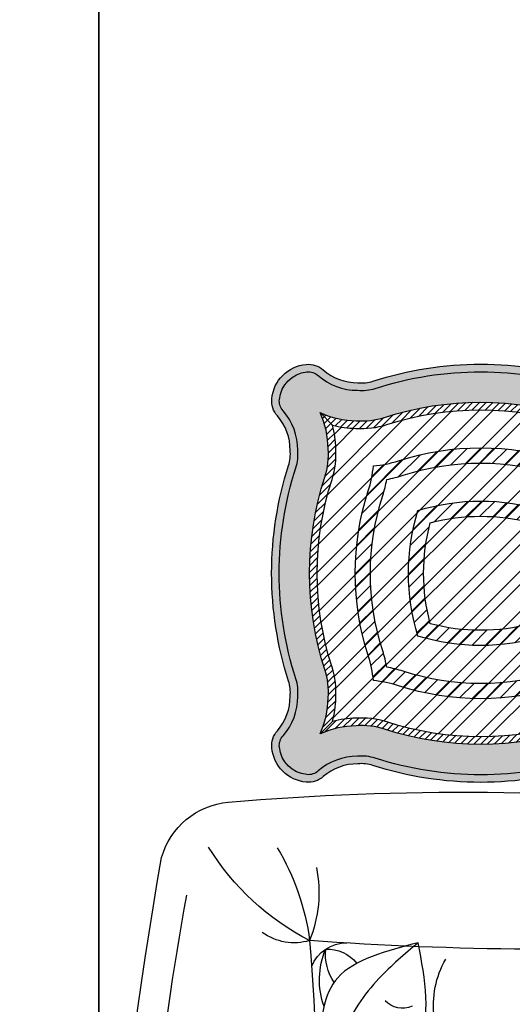
# Model space of a CAD drawing. Units: inches. Extents: x 844 to 2234, y 346 to 1084.
# Tile 23 of 93: x 1095 to 1105, y 710 to 731. Entities that reach past the tile are written whole.
import ezdxf

# ---------------------------------------------------------------- set-up
doc = ezdxf.new("R2010")
doc.units = ezdxf.units.IN
doc.header["$MEASUREMENT"] = 0
for name, color, linetype, lineweight in [('A-ANNO-DIMS', 2, 'Continuous', 18), ('A-WALL', 7, 'Continuous', 35), ('furniture', 8, 'Continuous', 18)]:
    doc.layers.add(name, color=color, linetype=linetype, lineweight=lineweight)
for name, color, linetype in [('RA-AP-01$0$FURN', 3, 'Continuous'), ('RA-AP-01$0$steel', 193, 'Continuous'), ('RA-AP-01$0$WOOD', 64, 'Continuous')]:
    doc.layers.add(name, color=color, linetype=linetype)
doc.styles.get("Standard").update_dxf_attribs({"font": 'arial.ttf'})
doc.dimstyles.get("Standard").update_dxf_attribs({"dimtxt": 6, "dimasz": 3, "dimexe": 0.18, "dimexo": 0.0625, "dimgap": 0.09, "dimtad": 0, "dimtih": 1, "dimtoh": 1, "dimdec": 1, "dimzin": 0, "dimdsep": 46, "dimlunit": 3, "dimtxsty": 'Standard', "dimblk": 'ARCHTICK', "dimcen": 0.09, "dimadec": 0, "dimazin": 0, "dimtfac": 1, "dimtdec": 1, "dimtofl": 0, "dimtmove": 0, "dimatfit": 3, "dimfxl": 1, "dimtolj": 1, "dimtzin": 0, "dimarcsym": 0})
pattern_1 = [(45, (0, 1.362436106329781), (-0.0088388347648318, 0.0088388347648318), [])]
pattern_2 = [(45, (0, 1.362436106329781), (-0.0044194173824159, 0.0044194173824159), [])]

# ---------------------------------------------------------------- blocks, each defined once
blk = doc.blocks.new('A$C2FCF5309')
at = {"layer": 'RA-AP-01$0$FURN'}
h = blk.add_hatch(dxfattribs=at)
h.set_pattern_fill('ANSI31', color=256, scale=0.1, style=0)
h.set_pattern_definition(pattern_1)
h.paths.add_polyline_path([(5.038683893313746, -5.169250834004607, -0.1583983521602212), (5.038683893312098, -5.373464580902012, 0.0306258898943267), (5.033304057242972, -5.394827569605182, 0.0306258898948892), (5.01194106853941, -5.40020740567441, -0.1028142994996694), (4.878286182323899, -5.414871334512708), (4.863600873530158, -5.43331743520547, 0.1120482678681049), (5.018059823131753, -5.419248541734471, -0.052642197802937), (5.050972078299936, -5.412495590662115, -0.0526421977994963), (5.057725029371615, -5.379583335496025, 0.1583028414702701), (5.057725029372958, -5.163132079409654, -0.052642197806903), (5.050972078299777, -5.130219824239078, -0.0526421977995126), (5.018059823133679, -5.123466873167369, 0.0215995840215353), (4.988903013548211, -5.115372132362452), (4.975007495303644, -5.132826183367946, -0.0289147572844802), (5.011941068537408, -5.142508009226167, 0.0306258898976746), (5.033304057242868, -5.147887845296027, 0.0306258899022411)])
h.paths.add_polyline_path([(4.975007495303645, -5.132826183367946), (4.988903013548211, -5.115372132362452, 0.1362374241599938), (4.801608567045604, -5.12346687316654, -0.0526421978036853), (4.768696311876971, -5.130219824239102, -0.05264219780204), (4.761943360804856, -5.163132079406747, 0.1583028414743723), (4.761943360806116, -5.379583335498449, -0.0526421977955461), (4.768696311877141, -5.412495590662114, -0.0526421978073986), (4.801608567048022, -5.419248541735437, 0.0454484293938888), (4.863600873530158, -5.43331743520547), (4.878286182323899, -5.414871334512708, -0.0546933379798044), (4.80772732164382, -5.40020740567649, 0.030625889903973), (4.786364332934043, -5.394827569605216, 0.0306258898932853), (4.780984496865101, -5.373464580902791, -0.1583983521638281), (4.780984496864308, -5.169250834000963, 0.03062588989692), (4.786364332933943, -5.147887845296004, 0.0306258898946324), (4.807727321637318, -5.142508009226805, -0.1288932573266927)])
h.paths.add_polyline_path([(4.843422214712861, -5.204945727074827, -0.0783685831716868), (4.924134454130224, -5.196727409635105), (4.939146578618322, -5.177870798323143, 0.1012675676854134), (4.827248748758957, -5.188772261120899, 0.1253648873081696), (4.820394258584192, -5.327034652050361), (4.837127701354095, -5.306015906404253, -0.0981593964869636)], flags=17)
h.paths.add_polyline_path([(4.843422214712824, -5.337769687826355, -0.0311091841722656), (4.837127701354095, -5.306015906404253), (4.820394258584193, -5.32703465205036, 0.0247727657431944), (4.827248748758908, -5.353943153780261, 0.0812754385032542), (4.916962478476905, -5.36629034358622), (4.933684093813825, -5.345286454285511, -0.0876255421014372)], flags=17)
h.paths.add_polyline_path([(4.992419641418037, -5.353943153780226, 0.1506053783834298), (4.992419641417933, -5.188772261120954, 0.0485966419124224), (4.939146578618321, -5.177870798323143), (4.924134454130224, -5.196727409635105, -0.0507799419579301), (4.976246175464031, -5.204945727074882, -0.1296645318906876), (4.97624617546411, -5.337769687826316, -0.0415667119298777), (4.933684093813825, -5.345286454285511), (4.916962478476905, -5.36629034358622, 0.0684915676023693)], flags=17)
h = blk.add_hatch(dxfattribs=at)
h.set_pattern_fill('ANSI31', color=256, scale=0.1, style=0)
h.set_pattern_definition(pattern_1)
h.paths.add_polyline_path([(5.038683893313746, -5.169250834004607, -0.1583983521602212), (5.038683893312098, -5.373464580902012, 0.0306258898943267), (5.033304057242972, -5.394827569605182, 0.0306258898948892), (5.01194106853941, -5.40020740567441, -0.1028142994996694), (4.878286182323899, -5.414871334512708), (4.863600873530158, -5.43331743520547, 0.1120482678681049), (5.018059823131753, -5.419248541734471, -0.052642197802937), (5.050972078299936, -5.412495590662115, -0.0526421977994963), (5.057725029371615, -5.379583335496025, 0.1583028414702701), (5.057725029372958, -5.163132079409654, -0.052642197806903), (5.050972078299777, -5.130219824239078, -0.0526421977995126), (5.018059823133679, -5.123466873167369, 0.0215995840215353), (4.988903013548211, -5.115372132362452), (4.975007495303644, -5.132826183367946, -0.0289147572844802), (5.011941068537408, -5.142508009226167, 0.0306258898976746), (5.033304057242868, -5.147887845296027, 0.0306258899022411)])
h.paths.add_polyline_path([(4.975007495303645, -5.132826183367946), (4.988903013548211, -5.115372132362452, 0.1362374241599938), (4.801608567045604, -5.12346687316654, -0.0526421978036853), (4.768696311876971, -5.130219824239102, -0.05264219780204), (4.761943360804856, -5.163132079406747, 0.1583028414743723), (4.761943360806116, -5.379583335498449, -0.0526421977955461), (4.768696311877141, -5.412495590662114, -0.0526421978073986), (4.801608567048022, -5.419248541735437, 0.0454484293938888), (4.863600873530158, -5.43331743520547), (4.878286182323899, -5.414871334512708, -0.0546933379798044), (4.80772732164382, -5.40020740567649, 0.030625889903973), (4.786364332934043, -5.394827569605216, 0.0306258898932853), (4.780984496865101, -5.373464580902791, -0.1583983521638281), (4.780984496864308, -5.169250834000963, 0.03062588989692), (4.786364332933943, -5.147887845296004, 0.0306258898946324), (4.807727321637318, -5.142508009226805, -0.1288932573266927)])
h.paths.add_polyline_path([(4.843422214712861, -5.204945727074827, -0.0783685831716868), (4.924134454130224, -5.196727409635105), (4.939146578618322, -5.177870798323143, 0.1012675676854134), (4.827248748758957, -5.188772261120899, 0.1253648873081696), (4.820394258584192, -5.327034652050361), (4.837127701354095, -5.306015906404253, -0.0981593964869636)], flags=17)
h.paths.add_polyline_path([(4.843422214712824, -5.337769687826355, -0.0311091841722656), (4.837127701354095, -5.306015906404253), (4.820394258584193, -5.32703465205036, 0.0247727657431944), (4.827248748758908, -5.353943153780261, 0.0812754385032542), (4.916962478476905, -5.36629034358622), (4.933684093813825, -5.345286454285511, -0.0876255421014372)], flags=17)
h.paths.add_polyline_path([(4.992419641418037, -5.353943153780226, 0.1506053783834298), (4.992419641417933, -5.188772261120954, 0.0485966419124224), (4.939146578618321, -5.177870798323143), (4.924134454130224, -5.196727409635105, -0.0507799419579301), (4.976246175464031, -5.204945727074882, -0.1296645318906876), (4.97624617546411, -5.337769687826316, -0.0415667119298777), (4.933684093813825, -5.345286454285511), (4.916962478476905, -5.36629034358622, 0.0684915676023693)], flags=17)
at = {"layer": 'RA-AP-01$0$WOOD'}
h = blk.add_hatch(color=256, dxfattribs=at)
edge = h.paths.add_edge_path()
edge.add_arc((4.683001772622394, -5.026441828662609), 0.0299999999999998, 48.77105092035535, 95.25687599427813)
edge.add_arc((4.684834195088484, -5.046357707450686), 0.0499999999998897, 95.25687599443106, 174.7431240064049)
edge.add_arc((4.664918316300367, -5.044525284985046), 0.0300000000000005, 174.7431240062535, 221.2289490796905)
edge.add_arc((4.591236830209155, -5.109094338216345), 0.0679700159630267, -0.5333070513215148, 41.228949079691915, ccw=False)
edge.add_arc((4.609451302807284, -5.114694777173187), 0.0500000000000008, -17.3556839752095, 5.7020707654044145, ccw=False)
edge.add_arc((5.095208119646659, -5.271357707450659), 0.4603971832811796, 162.0683908477609, 197.9316091523306)
edge.add_arc((4.609451302807533, -5.428020637728902), 0.0500000000000006, -5.702070765320514, 17.355683975293914, ccw=False)
edge.add_arc((4.591236830209412, -5.433621076685779), 0.0679700159630261, -41.228949079600625, 0.5333070514128053, ccw=False)
edge.add_arc((4.664918316300727, -5.498190129916959), 0.0299999999999995, 138.7710509204022, 185.256875994324)
edge.add_arc((4.684834195088642, -5.496357707450695), 0.0499999999997451, 185.2568759946742, 264.74312400432)
edge.add_arc((4.683001772622394, -5.516273586238612), 0.03, 264.743124003969, 311.2289490796446)
edge.add_arc((4.747570825853633, -5.589955072329876), 0.0679700159630271, 89.4666929486321, 131.2289490796457, ccw=False)
edge.add_arc((4.753171264810493, -5.57174059973175), 0.0500000000000015, 72.64431602474701, 95.70207076536133, ccw=False)
edge.add_arc((4.909834195088355, -5.085983782892503), 0.4603971832811774, 252.0683908477147, 287.9316091522845)
edge.add_arc((5.06649712536621, -5.57174059973175), 0.0499999999999999, 84.29792923463953, 107.35568397525361, ccw=False)
edge.add_arc((5.072097564323069, -5.589955072329877), 0.0679700159630274, 48.771050920354185, 90.5333070513679, ccw=False)
edge.add_arc((5.136666617554309, -5.516273586238614), 0.0299999999999997, 228.771050920353, 275.2568759942969)
edge.add_arc((5.134834195088338, -5.496357707450417), 0.0499999999999982, 275.2568759942949, 354.7431240057633)
edge.add_arc((5.154750073876535, -5.498190129916372), 0.0299999999999999, 354.7431240057662, 401.2289490796891)
edge.add_arc((5.228431559967749, -5.433621076685074), 0.0679700159630274, 179.4666929486771, 221.2289490796903, ccw=False)
edge.add_arc((5.210217087369615, -5.428020637728227), 0.0499999999999976, 162.6443160247947, 185.7020707654089, ccw=False)
edge.add_arc((4.724460270530244, -5.271357707450757), 0.4603971832811793, 342.0683908477607, 377.9316091523305)
edge.add_arc((5.210217087369368, -5.114694777172509), 0.0500000000000019, 174.2979292346878, 197.355683975302, ccw=False)
edge.add_arc((5.228431559967489, -5.109094338215639), 0.0679700159630279, 138.7710509203993, 180.5333070514128, ccw=False)
edge.add_arc((5.154750073876174, -5.044525284984457), 0.0300000000000001, 318.771050920401, 365.2568759954636)
edge.add_arc((5.13483419508816, -5.046357707450624), 0.0499999999998349, 5.256875995237118, 84.74312400549572)
edge.add_arc((5.136666617554308, -5.026441828662608), 0.0299999999999994, 84.74312400572185, 131.2289490796446)
edge.add_arc((5.072097564323072, -4.952760342571343), 0.0679700159630261, 269.4666929486298, 311.22894907964354, ccw=False)
edge.add_arc((5.066497125366206, -4.97097481516947), 0.0499999999999992, 252.64431602475162, 275.70207076536565, ccw=False)
edge.add_arc((4.909834195088355, -5.456731632008717), 0.4603971832811764, 72.06839084771546, 107.9316091522853)
edge.add_arc((4.753171264810493, -4.970974815169471), 0.0500000000000016, 264.2979292346387, 287.355683975253, ccw=False)
edge.add_arc((4.747570825853633, -4.952760342571346), 0.0679700159630274, 228.7710509203543, 270.5333070513679, ccw=False)
edge = h.paths.add_edge_path(flags=16)
edge.add_arc((4.683001772622395, -5.026441828662608), 0.019999999999999, 48.7710509203555, 95.2568759942793)
edge.add_arc((4.684834195088469, -5.046357707450671), 0.0399999999998731, 95.2568759944489, 174.7431240064248)
edge.add_arc((4.664918316300404, -5.044525284985035), 0.020000000000036, 174.7431240062186, 221.2289490796461)
edge.add_arc((4.591236830209151, -5.109094338216346), 0.0779700159630296, -0.13764630038667747, 41.228949079689585, ccw=False)
edge.add_arc((4.609451302807307, -5.11469477717304), 0.060000000000024, -17.406127045137907, 5.176192161068002, ccw=False)
edge.add_arc((5.09520811964665, -5.271357707450659), 0.4503971832811708, 162.0623235129628, 197.9376764869162)
edge.add_arc((4.609451302807532, -5.428020637728943), 0.0599999999999982, -5.176192160466428, 17.406127046715312, ccw=False)
edge.add_arc((4.591236830209414, -5.433621076685778), 0.0779700159630257, -41.2289490796029, 0.13764630095249686, ccw=False)
edge.add_arc((4.664918316300731, -5.498190129916961), 0.0200000000000047, 138.7710509204103, 185.2568759943212)
edge.add_arc((4.684834195088606, -5.496357707450731), 0.0399999999997066, 185.2568759947174, 264.7431240043665)
edge.add_arc((4.683001772622369, -5.516273586238541), 0.020000000000069, 264.7431240038842, 311.2289490795622)
edge.add_arc((4.747570825853635, -5.589955072329884), 0.0779700159630344, 89.8623536987642, 131.2289490796432, ccw=False)
edge.add_arc((4.753171264810603, -5.571740599731771), 0.0599999999999895, 72.5938729544394, 95.1761921602253, ccw=False)
edge.add_arc((4.909834195088365, -5.085983782892505), 0.4503971832811724, 252.0623235129989, 287.9376764870498)
edge.add_arc((5.066497125366216, -5.571740599731755), 0.0600000000000047, 84.8238078399923, 107.40612704528041, ccw=False)
edge.add_arc((5.072097564322998, -5.589955072329853), 0.077970015963056, 48.771050920303594, 90.13764630126451, ccw=False)
edge.add_arc((5.136666617554307, -5.516273586238622), 0.0199999999999931, 228.771050920344, 275.2568759943037)
edge.add_arc((5.134834195088338, -5.496357707450416), 0.0400000000000004, 275.2568759942928, 354.7431240057607)
edge.add_arc((5.154750073876533, -5.498190129916375), 0.0200000000000037, 354.7431240057783, 401.2289490796939)
edge.add_arc((5.228431559967745, -5.433621076685076), 0.0779700159630239, 179.8623536995147, 221.2289490796908, ccw=False)
edge.add_arc((5.210217087369586, -5.428020637728345), 0.0600000000000054, 162.5938729554486, 185.1761921609759, ccw=False)
edge.add_arc((4.724460270530243, -5.271357707450766), 0.4503971832811826, 342.0623235128896, 377.937676486982)
edge.add_arc((5.210217087369347, -5.114694777172486), 0.0599999999999777, 174.8238078387611, 197.4061270462219, ccw=False)
edge.add_arc((5.228431559967523, -5.109094338215542), 0.0779700159629885, 138.7710509204687, 180.1376463004423, ccw=False)
edge.add_arc((5.154750073876175, -5.044525284984459), 0.0199999999999989, 318.771050920406, 365.2568759954698)
edge.add_arc((5.134834195088138, -5.046357707450646), 0.0399999999998586, 5.256875995208452, 84.74312400546732)
edge.add_arc((5.136666617554292, -5.02644182866256), 0.0199999999999529, 84.74312400577769, 131.2289490797025)
edge.add_arc((5.072097564323069, -4.952760342571338), 0.077970015963032, 269.86235369901414, 311.2289490796421, ccw=False)
edge.add_arc((5.06649712536618, -4.97097481516946), 0.0600000000000007, 252.5938729548277, 275.17619216047467, ccw=False)
edge.add_arc((4.909834195088353, -5.456731632008716), 0.4503971832811739, 72.06232351293887, 107.9376764867365)
edge.add_arc((4.753171264810429, -4.970974815169467), 0.0599999999999991, 264.82380783985815, 287.40612704769893, ccw=False)
edge.add_arc((4.747570825853681, -4.952760342571361), 0.0779700159630467, 228.7710509203206, 270.13764630113724, ccw=False)
h = blk.add_hatch(color=256, dxfattribs=at)
edge = h.paths.add_edge_path()
edge.add_arc((4.683001772622395, -5.026441828662608), 0.019999999999999, 48.7710509203555, 95.2568759942793)
edge.add_arc((4.684834195088469, -5.046357707450671), 0.0399999999998731, 95.2568759944489, 174.7431240064248)
edge.add_arc((4.664918316300404, -5.044525284985035), 0.020000000000036, 174.7431240062186, 221.2289490796461)
edge.add_arc((4.591236830209151, -5.109094338216346), 0.0779700159630296, -0.13764630038667747, 41.228949079689585, ccw=False)
edge.add_arc((4.609451302807307, -5.11469477717304), 0.060000000000024, -17.406127045137907, 5.176192161068002, ccw=False)
edge.add_arc((5.09520811964665, -5.271357707450659), 0.4503971832811708, 162.0623235129628, 197.9376764869162)
edge.add_arc((4.609451302807532, -5.428020637728943), 0.0599999999999982, -5.176192160466428, 17.406127046715312, ccw=False)
edge.add_arc((4.591236830209414, -5.433621076685778), 0.0779700159630257, -41.2289490796029, 0.13764630095249686, ccw=False)
edge.add_arc((4.664918316300731, -5.498190129916961), 0.0200000000000047, 138.7710509204103, 185.2568759943212)
edge.add_arc((4.684834195088606, -5.496357707450731), 0.0399999999997066, 185.2568759947174, 264.7431240043665)
edge.add_arc((4.683001772622369, -5.516273586238541), 0.020000000000069, 264.7431240038842, 311.2289490795622)
edge.add_arc((4.747570825853635, -5.589955072329884), 0.0779700159630344, 89.8623536987642, 131.2289490796432, ccw=False)
edge.add_arc((4.753171264810603, -5.571740599731771), 0.0599999999999895, 72.5938729544394, 95.1761921602253, ccw=False)
edge.add_arc((4.909834195088365, -5.085983782892505), 0.4503971832811724, 252.0623235129989, 287.9376764870498)
edge.add_arc((5.066497125366216, -5.571740599731755), 0.0600000000000047, 84.8238078399923, 107.40612704528041, ccw=False)
edge.add_arc((5.072097564322998, -5.589955072329853), 0.077970015963056, 48.771050920303594, 90.13764630126451, ccw=False)
edge.add_arc((5.136666617554307, -5.516273586238622), 0.0199999999999931, 228.771050920344, 275.2568759943037)
edge.add_arc((5.134834195088338, -5.496357707450416), 0.0400000000000004, 275.2568759942928, 354.7431240057607)
edge.add_arc((5.154750073876533, -5.498190129916375), 0.0200000000000037, 354.7431240057783, 401.2289490796939)
edge.add_arc((5.228431559967745, -5.433621076685076), 0.0779700159630239, 179.8623536995147, 221.2289490796908, ccw=False)
edge.add_arc((5.210217087369586, -5.428020637728345), 0.0600000000000054, 162.5938729554486, 185.1761921609759, ccw=False)
edge.add_arc((4.724460270530243, -5.271357707450766), 0.4503971832811826, 342.0623235128896, 377.937676486982)
edge.add_arc((5.210217087369347, -5.114694777172486), 0.0599999999999777, 174.8238078387611, 197.4061270462219, ccw=False)
edge.add_arc((5.228431559967523, -5.109094338215542), 0.0779700159629885, 138.7710509204687, 180.1376463004423, ccw=False)
edge.add_arc((5.154750073876175, -5.044525284984459), 0.0199999999999989, 318.771050920406, 365.2568759954698)
edge.add_arc((5.134834195088138, -5.046357707450646), 0.0399999999998586, 5.256875995208452, 84.74312400546732)
edge.add_arc((5.136666617554292, -5.02644182866256), 0.0199999999999529, 84.74312400577769, 131.2289490797025)
edge.add_arc((5.072097564323069, -4.952760342571338), 0.077970015963032, 269.86235369901414, 311.2289490796421, ccw=False)
edge.add_arc((5.06649712536618, -4.97097481516946), 0.0600000000000007, 252.5938729548277, 275.17619216047467, ccw=False)
edge.add_arc((4.909834195088353, -5.456731632008716), 0.4503971832811739, 72.06232351293887, 107.9376764867365)
edge.add_arc((4.753171264810429, -4.970974815169467), 0.0599999999999991, 264.82380783985815, 287.40612704769893, ccw=False)
edge.add_arc((4.747570825853681, -4.952760342571361), 0.0779700159630467, 228.7710509203206, 270.13764630113724, ccw=False)
edge = h.paths.add_edge_path(flags=16)
edge.add_arc((4.591236830209151, -5.109094338216348), 0.1179700159630308, 0.7417751874182841, 24.563326950263672, ccw=False)
edge.add_arc((4.609451302807302, -5.114694777173093), 0.100000000000012, -17.52836504564658, 4.087328884225087, ccw=False)
edge.add_arc((5.095208119646651, -5.271357707450657), 0.4103971832811724, 162.0403002448777, 197.9596997550675)
edge.add_arc((4.60945130280753, -5.428020637728918), 0.1000000000000027, -4.087328883827581, 17.528365046291924, ccw=False)
edge.add_arc((4.591236830209414, -5.433621076685779), 0.1179700159630246, 335.43667305041845, 359.2582248129738, ccw=False)
edge.add_arc((4.747570825853596, -5.589955072329891), 0.117970015963042, 90.7417751868461, 114.5633269496104, ccw=False)
edge.add_arc((4.753171264810559, -5.571740599731767), 0.0999999999999976, 72.47163495370341, 94.0873288836737, ccw=False)
edge.add_arc((4.909834195088367, -5.085983782892503), 0.4103971832811735, 252.0403002449999, 287.9596997551833)
edge.add_arc((5.066497125366205, -5.571740599731755), 0.1000000000000057, 85.91267111645209, 107.5283650455624, ccw=False)
edge.add_arc((5.072097564322985, -5.58995507232986), 0.117970015963046, 65.4366730497672, 89.25822481317113, ccw=False)
edge.add_arc((5.22843155996773, -5.433621076684992), 0.1179700159630096, 180.7417751873964, 204.5633269502712, ccw=False)
edge.add_arc((5.210217087369591, -5.428020637728301), 0.0999999999999969, 162.4716349546276, 184.0873288841682, ccw=False)
edge.add_arc((4.724460270530243, -5.271357707450766), 0.4103971832811825, 342.0403002448147, 377.9596997550345)
edge.add_arc((5.210217087369347, -5.114694777172489), 0.0999999999999796, 175.9126711156995, 197.5283650464392, ccw=False)
edge.add_arc((5.228431559967512, -5.109094338215525), 0.1179700159630019, 155.4366730502992, 179.2582248126247, ccw=False)
edge.add_arc((5.072097564323172, -4.952760342571314), 0.1179700159630537, 270.74177518697286, 294.56332694975765, ccw=False)
edge.add_arc((5.066497125366189, -4.970974815169462), 0.1000000000000017, 252.471634954247, 274.0873288838353, ccw=False)
edge.add_arc((4.909834195088353, -5.456731632008716), 0.4103971832811758, 72.04030024486342, 107.9596997549354)
edge.add_arc((4.75317126481046, -4.970974815169467), 0.1000000000000041, 265.91267111635307, 287.5283650466103, ccw=False)
edge.add_arc((4.747570825853629, -4.952760342571342), 0.1179700159630538, 245.43667304992562, 269.2582248131125, ccw=False)
h = blk.add_hatch(dxfattribs=at)
h.set_pattern_fill('ANSI31', color=256, scale=0.05, style=0)
h.set_pattern_definition(pattern_2)
h.paths.add_polyline_path([(5.105336294329346, -5.394854099602528, 0.0940138826956367), (5.100476366643778, -5.435568764288975, 0.0606271852326483), (5.104678567100611, -5.466202079462671, 0.0606271852344644), (5.074045251925975, -5.46199987900586, 0.0940138827021426), (5.033330587236848, -5.466859806692645, -0.1305325492494615), (4.828072633169377, -5.477944178050054), (4.821119726105699, -5.486677669841435, 0.1336226599878005), (5.036379334063467, -5.476383803188216, -0.0945969211935747), (5.073624810952389, -5.471994942692536, -0.1043170707892296), (5.121137550891356, -5.48266106325342, -0.1043170707868944), (5.110471430330457, -5.435148323315565, -0.0945969211952573), (5.114860290825935, -5.397902846425963, 0.1580239521433527), (5.114860290826324, -5.144812568476775, -0.0945969212010491), (5.110471430330247, -5.10756709158498, -0.1043170707844371), (5.121137550890657, -5.060054351648168, -0.104317070786514), (5.073624810952866, -5.070720472208642, -0.0945969211958523), (5.036379334063063, -5.066331611712874, 0.1580239521426795), (4.783289056114906, -5.066331611712465, -0.0945969211985319), (4.746043579224103, -5.070720472208672, -0.1043170707882665), (4.698530839285552, -5.060054351647925, -0.1043170707867205), (4.709196959846443, -5.10756709158571, -0.094596921196788), (4.704808099350826, -5.144812568475902, 0.1580239521433127), (4.704808099350699, -5.397902846425022, -0.094596921197841), (4.709196959846712, -5.435148323315576, -0.1043170707855109), (4.698530839286393, -5.482661063252921, -0.1043170707864168), (4.746043579224162, -5.471994942692571, -0.0945969211977586), (4.783289056114671, -5.476383803188671, 0.0238966994662183), (4.821119726105699, -5.486677669841435), (4.828072633169378, -5.477944178050054, -0.0269814195959459), (4.786337802940177, -5.466859806692736, 0.0940138827039629), (4.745623138250268, -5.461999879005895, 0.0606271852320776), (4.714989823076826, -5.466202079462476, 0.0606271852304618), (4.719192023533341, -5.435568764289856, 0.0940138826917763), (4.714332095848404, -5.394854099604977, -0.1580706864542086), (4.714332095846561, -5.147861315302034, 0.0940138827032017), (4.719192023533127, -5.107146650612438, 0.0606271852329446), (4.714989823076289, -5.076513335438588, 0.0606271852340035), (4.745623138250698, -5.08071553589536, 0.0940138827025969), (4.786337802940015, -5.075855608208526, -0.1580706864508517), (5.033330587237968, -5.075855608208939, 0.0940138827009578), (5.074045251926627, -5.080715535895319, 0.0606271852322557), (5.104678567100159, -5.076513335438697, 0.0606271852308743), (5.100476366643561, -5.107146650611519, 0.0940138827178109), (5.105336294331983, -5.147861315307182, -0.1580706864490946)])
h = blk.add_hatch(dxfattribs=at)
h.set_pattern_fill('ANSI31', color=256, scale=0.05, style=0)
h.set_pattern_definition(pattern_2)
h.paths.add_polyline_path([(5.105336294329346, -5.394854099602528, 0.0940138826956367), (5.100476366643778, -5.435568764288975, 0.0606271852326483), (5.104678567100611, -5.466202079462671, 0.0606271852344644), (5.074045251925975, -5.46199987900586, 0.0940138827021426), (5.033330587236848, -5.466859806692645, -0.1305325492494615), (4.828072633169377, -5.477944178050054), (4.821119726105699, -5.486677669841435, 0.1336226599878005), (5.036379334063467, -5.476383803188216, -0.0945969211935747), (5.073624810952389, -5.471994942692536, -0.1043170707892296), (5.121137550891356, -5.48266106325342, -0.1043170707868944), (5.110471430330457, -5.435148323315565, -0.0945969211952573), (5.114860290825935, -5.397902846425963, 0.1580239521433527), (5.114860290826324, -5.144812568476775, -0.0945969212010491), (5.110471430330247, -5.10756709158498, -0.1043170707844371), (5.121137550890657, -5.060054351648168, -0.104317070786514), (5.073624810952866, -5.070720472208642, -0.0945969211958523), (5.036379334063063, -5.066331611712874, 0.1580239521426795), (4.783289056114906, -5.066331611712465, -0.0945969211985319), (4.746043579224103, -5.070720472208672, -0.1043170707882665), (4.698530839285552, -5.060054351647925, -0.1043170707867205), (4.709196959846443, -5.10756709158571, -0.094596921196788), (4.704808099350826, -5.144812568475902, 0.1580239521433127), (4.704808099350699, -5.397902846425022, -0.094596921197841), (4.709196959846712, -5.435148323315576, -0.1043170707855109), (4.698530839286393, -5.482661063252921, -0.1043170707864168), (4.746043579224162, -5.471994942692571, -0.0945969211977586), (4.783289056114671, -5.476383803188671, 0.0238966994662183), (4.821119726105699, -5.486677669841435), (4.828072633169378, -5.477944178050054, -0.0269814195959459), (4.786337802940177, -5.466859806692736, 0.0940138827039629), (4.745623138250268, -5.461999879005895, 0.0606271852320776), (4.714989823076826, -5.466202079462476, 0.0606271852304618), (4.719192023533341, -5.435568764289856, 0.0940138826917763), (4.714332095848404, -5.394854099604977, -0.1580706864542086), (4.714332095846561, -5.147861315302034, 0.0940138827032017), (4.719192023533127, -5.107146650612438, 0.0606271852329446), (4.714989823076289, -5.076513335438588, 0.0606271852340035), (4.745623138250698, -5.08071553589536, 0.0940138827025969), (4.786337802940015, -5.075855608208526, -0.1580706864508517), (5.033330587237968, -5.075855608208939, 0.0940138827009578), (5.074045251926627, -5.080715535895319, 0.0606271852322557), (5.104678567100159, -5.076513335438697, 0.0606271852308743), (5.100476366643561, -5.107146650611519, 0.0940138827178109), (5.105336294331983, -5.147861315307182, -0.1580706864490946)])
h = blk.add_hatch(dxfattribs=at)
h.set_pattern_fill('ANSI32,_I', color=256, scale=0.1, style=2)
h.set_pattern_definition([(45, (0, 0), (-0.0265165042944955, 0.0265165042944955), []), (45, (0.0176776695, 0), (-0.0265165042944955, 0.0265165042944955), [])])
h.paths.add_polyline_path([(4.843422214712824, -5.337769687826354, 0.1296645318905289), (4.97624617546411, -5.337769687826316, 0.1296645318906876), (4.976246175464032, -5.204945727074882, 0.129664531890418), (4.843422214712861, -5.204945727074827, 0.129664531890765)], flags=0)
h.paths.add_polyline_path([(5.039131224122924, -5.170637849998464, -0.0326520429852175), (5.033304057242868, -5.147887845296027, -0.0326520429894721), (5.010554052537512, -5.142060678415043, 0.1561383235202698), (4.809114337641437, -5.142060678414318, -0.0326520429925972), (4.786364332933944, -5.147887845296004, -0.0326520429914489), (4.780537166052582, -5.170637850002729, 0.1561383235189577), (4.780537166052134, -5.37207756489719, -0.0326520429934175), (4.786364332934042, -5.394827569605215, -0.0326520429823496), (4.809114337634529, -5.400654736484653, 0.156138323524066), (5.010554052535268, -5.400654736486903, -0.032652042992888), (5.033304057242972, -5.394827569605183, -0.0326520429928733), (5.039131224124712, -5.372077564897496, 0.1561383235226786)], flags=0)
h.paths.add_polyline_path([(4.992419641418037, -5.353943153780226, -0.1506053783832862), (4.827248748758909, -5.353943153780261, -0.1506053783835069), (4.827248748758957, -5.188772261120899, -0.1506053783831346), (4.992419641417933, -5.188772261120954, -0.1506053783834298)], flags=0)
h.paths.add_polyline_path([(4.976246175464111, -5.337769687826316, -0.1296645318905298), (4.843422214712824, -5.337769687826354, -0.129664531890765), (4.843422214712862, -5.204945727074827, -0.1296645318904162), (4.976246175464031, -5.204945727074882, -0.1296645318906876)], flags=0)
h.paths.add_polyline_path([(5.105721254232479, -5.149054940982025, -0.0968902512052664), (5.100476366643561, -5.107146650611519, -0.0606271852308743), (5.104678567100159, -5.076513335438697, -0.0606271852322574), (5.074045251926626, -5.080715535895319, -0.0968902512197216), (5.032136961550132, -5.075470648304253, 0.1564657949319774), (4.787531428625239, -5.075470648304682, -0.0968902512150626), (4.745623138250699, -5.08071553589536, -0.060627185234009), (4.714989823076288, -5.076513335438587, -0.0606271852329501), (4.719192023533127, -5.10714665061244, -0.0968902512185585), (4.713947135942331, -5.149054940988458, 0.1564657949285579), (4.713947135940853, -5.393660473908259, -0.0968902512319826), (4.71919202353334, -5.435568764289873, -0.0606271852304288), (4.714989823076825, -5.466202079462476, -0.0606271852320811), (4.745623138250269, -5.461999879005895, -0.0968902512162649), (4.787531428625332, -5.467244766596559, 0.1564657949327057), (5.032136961551311, -5.46724476659659, -0.0968902512153659), (5.074045251925975, -5.46199987900586, -0.0606271852344627), (5.10467856710061, -5.466202079462671, -0.0606271852326483), (5.100476366643777, -5.435568764288975, -0.0968902512258216), (5.105721254235559, -5.393660473909953, 0.1564657949340142)])
h.paths.add_polyline_path([(5.057725029371625, -5.379583335495999, 0.0526421977995391), (5.050972078299936, -5.412495590662114, 0.0526421978029782), (5.018059823131728, -5.419248541734479, -0.1583028414681072), (4.801608567048168, -5.419248541735485, 0.0526421978076402), (4.76869631187714, -5.412495590662113, 0.0526421977956189), (4.761943360806101, -5.379583335498404, -0.1583028414743129), (4.761943360804846, -5.163132079406778, 0.0526421978020944), (4.768696311876972, -5.130219824239101, 0.0526421978033651), (4.80160856704541, -5.123466873166602, -0.1583028414716875), (5.018059823133628, -5.123466873167353, 0.0526421977995944), (5.050972078299776, -5.130219824239078, 0.0526421978070423), (5.057725029372986, -5.163132079409739, -0.1583028414701848)], flags=16)
h.paths.add_polyline_path([(5.038683893312112, -5.373464580901968, 0.0306258898943915), (5.033304057242972, -5.394827569605182, 0.0306258898948892), (5.01194106853941, -5.40020740567441, -0.1583983521587032), (4.807727321643864, -5.400207405676503, 0.0306258899040366), (4.786364332934043, -5.394827569605215, 0.0306258898931986), (4.780984496865119, -5.37346458090285, -0.1583983521638542), (4.7809844968643, -5.169250834000989, 0.0306258898969596), (4.786364332933945, -5.147887845296004, 0.0306258898946195), (4.807727321637311, -5.142508009226808, -0.1583983521623412), (5.011941068537318, -5.142508009226139, 0.030625889897807), (5.033304057242868, -5.147887845296028, 0.0306258899020632), (5.038683893313706, -5.169250834004486, -0.1583983521602835)], flags=0)
for p, q in [((4.714989823076289, -5.076513335438588), (4.698530839285552, -5.060054351647925)), ((4.714989823076289, -5.076513335438588), (4.698530839285552, -5.060054351647925)), ((5.104678567100159, -5.076513335438697), (5.121137550890656, -5.060054351648169)), ((5.104678567100159, -5.076513335438697), (5.121137550890656, -5.060054351648169)), ((5.10467856710061, -5.466202079462671), (5.121137550891355, -5.482661063253419)), ((5.10467856710061, -5.466202079462671), (5.121137550891355, -5.482661063253419))]:
    blk.add_line(p, q, dxfattribs=at)
for points in [[(4.702773858784635, -5.003879368495489, 0.2056608120285223), (4.680253138923443, -4.996568010480312, 0.3614336704708569), (4.635044498118043, -5.041776651286372, 0.2056608120263112), (4.642355856133262, -5.064297371147306, -0.1842662638101064), (4.65920390179375, -5.10972699154053, -0.1009492694051416), (4.657174869772992, -5.129609908955028, 0.1577727036674954), (4.657174869773219, -5.41310550594699, -0.1009492694051416), (4.659203901794006, -5.432988423361486, -0.1842662638101064), (4.64235585613359, -5.478418043754737, 0.2056608120285221), (4.635044498118431, -5.500938763615934, 0.3614336704593693), (4.680253138922529, -5.546147404420826, 0.2056608120364936), (4.702773858784635, -5.538836046405732, -0.1842662638101064), (4.748203479177874, -5.52198800074528, -0.1009492694051415), (4.768086396592371, -5.524017032766053, 0.1577727036674954), (5.051581993584332, -5.524017032766055, -0.1009492694051416), (5.071464910998829, -5.521988000745282, -0.1842662638101064), (5.116894531392067, -5.538836046405734, 0.2056608120286145), (5.13941525125327, -5.546147404420911, 0.3614336704683636), (5.184623892058835, -5.500938763615299, 0.2056608120285223), (5.177312534043641, -5.478418043754112, -0.1842662638101063), (5.160464488383153, -5.432988423360887, -0.1009492694051416), (5.162493520403909, -5.41310550594639, 0.1577727036674954), (5.162493520403684, -5.129609908954428, -0.1009492694051416), (5.160464488382894, -5.109726991539933, -0.1842662638101064), (5.17731253404331, -5.064297371146681, 0.2056608120337072), (5.184623892058415, -5.041776651284888, 0.3614336704623863), (5.139415251253259, -4.99656801048031, 0.2056608120285223), (5.116894531392067, -5.003879368495487, -0.1842662638101064), (5.071464910998829, -5.020727414155937, -0.1009492694051416), (5.051581993584332, -5.018698382135166, 0.1577727036674956), (4.768086396592371, -5.018698382135168, -0.1009492694051416), (4.748203479177874, -5.020727414155941, -0.1842662638101064)], [(4.702773858784635, -5.003879368495489, 0.2056608120285223), (4.680253138923443, -4.996568010480312, 0.3614336704708569), (4.635044498118043, -5.041776651286372, 0.2056608120263112), (4.642355856133262, -5.064297371147306, -0.1842662638101064), (4.65920390179375, -5.10972699154053, -0.1009492694051416), (4.657174869772992, -5.129609908955028, 0.1577727036674954), (4.657174869773219, -5.41310550594699, -0.1009492694051416), (4.659203901794006, -5.432988423361486, -0.1842662638101064), (4.64235585613359, -5.478418043754737, 0.2056608120285221), (4.635044498118431, -5.500938763615934, 0.3614336704593693), (4.680253138922529, -5.546147404420826, 0.2056608120364936), (4.702773858784635, -5.538836046405732, -0.1842662638101064), (4.748203479177874, -5.52198800074528, -0.1009492694051415), (4.768086396592371, -5.524017032766053, 0.1577727036674954), (5.051581993584332, -5.524017032766055, -0.1009492694051416), (5.071464910998829, -5.521988000745282, -0.1842662638101064), (5.116894531392067, -5.538836046405734, 0.2056608120286145), (5.13941525125327, -5.546147404420911, 0.3614336704683636), (5.184623892058835, -5.500938763615299, 0.2056608120285223), (5.177312534043641, -5.478418043754112, -0.1842662638101063), (5.160464488383153, -5.432988423360887, -0.1009492694051416), (5.162493520403909, -5.41310550594639, 0.1577727036674954), (5.162493520403684, -5.129609908954428, -0.1009492694051416), (5.160464488382894, -5.109726991539933, -0.1842662638101064), (5.17731253404331, -5.064297371146681, 0.2056608120337072), (5.184623892058415, -5.041776651284888, 0.3614336704623863), (5.139415251253259, -4.99656801048031, 0.2056608120285223), (5.116894531392067, -5.003879368495487, -0.1842662638101064), (5.071464910998829, -5.020727414155937, -0.1009492694051416), (5.051581993584332, -5.018698382135166, 0.1577727036674956), (4.768086396592371, -5.018698382135168, -0.1009492694051416), (4.748203479177874, -5.020727414155941, -0.1842662638101064)], [(4.696183163397222, -5.011400188551196, 0.2056608120285295), (4.681169350156427, -5.006525949874411, 0.3614336704708588), (4.645002437512154, -5.042692862519237, 0.2056608120262659), (4.649876676188964, -5.057706675759887, -0.182481815856965), (4.669206621172843, -5.109281651732388, -0.0988540857970112), (4.666703803477437, -5.13264334722805, 0.1578269695851905), (4.666703803477144, -5.410072067672365, -0.0988540858013112), (4.6692066211731, -5.433433763168966, -0.1824818158591246), (4.649876676189301, -5.485008739142145, 0.2056608120284717), (4.64500243751253, -5.500022552382944, 0.3614336704593821), (4.681169350155757, -5.536189465026749, 0.2056608120365057), (4.696183163397221, -5.531315226350026, -0.1824818158605826), (4.747758139370833, -5.51198528136619, -0.0988540857951607), (4.771119834866025, -5.514488099061806, 0.1578269695856264), (5.04854855531107, -5.514488099061688, -0.0988540857929677), (5.071910250805761, -5.511985281366138, -0.1824818158609529), (5.123485226779481, -5.531315226350027, 0.2056608120286893), (5.138499040020282, -5.536189465026812, 0.3614336704683556), (5.174665952664737, -5.500022552382323, 0.2056608120284882), (5.169791713987938, -5.485008739141532, -0.1824818158574124), (5.150461769004059, -5.4334337631689, -0.0988540857940221), (5.152964586699289, -5.410072067673927, 0.1578269695858123), (5.1529645866996, -5.132643347228565, -0.0988540858025403), (5.150461769003872, -5.109281651731659, -0.1824818158565006), (5.169791713987599, -5.057706675759273, 0.2056608120337192), (5.174665952664335, -5.042692862518078, 0.3614336704623903), (5.138499040020236, -5.006525949874406, 0.2056608120285323), (5.123485226779481, -5.011400188551195, -0.1824818158594503), (5.071910250806212, -5.03073013353503, -0.09885408579455), (5.048548555311143, -5.028227315839558, 0.1578269695844942), (4.771119834867991, -5.028227315838772, -0.0988540858042156), (4.747758139370745, -5.030730133535067, -0.1824818158603032)], [(4.696183163397222, -5.011400188551196, 0.2056608120285295), (4.681169350156427, -5.006525949874411, 0.3614336704708588), (4.645002437512154, -5.042692862519237, 0.2056608120262659), (4.649876676188964, -5.057706675759887, -0.182481815856965), (4.669206621172843, -5.109281651732388, -0.0988540857970112), (4.666703803477437, -5.13264334722805, 0.1578269695851905), (4.666703803477144, -5.410072067672365, -0.0988540858013112), (4.6692066211731, -5.433433763168966, -0.1824818158591246), (4.649876676189301, -5.485008739142145, 0.2056608120284717), (4.64500243751253, -5.500022552382944, 0.3614336704593821), (4.681169350155757, -5.536189465026749, 0.2056608120365057), (4.696183163397221, -5.531315226350026, -0.1824818158605826), (4.747758139370833, -5.51198528136619, -0.0988540857951607), (4.771119834866025, -5.514488099061806, 0.1578269695856264), (5.04854855531107, -5.514488099061688, -0.0988540857929677), (5.071910250805761, -5.511985281366138, -0.1824818158609529), (5.123485226779481, -5.531315226350027, 0.2056608120286893), (5.138499040020282, -5.536189465026812, 0.3614336704683556), (5.174665952664737, -5.500022552382323, 0.2056608120284882), (5.169791713987938, -5.485008739141532, -0.1824818158574124), (5.150461769004059, -5.4334337631689, -0.0988540857940221), (5.152964586699289, -5.410072067673927, 0.1578269695858123), (5.1529645866996, -5.132643347228565, -0.0988540858025403), (5.150461769003872, -5.109281651731659, -0.1824818158565006), (5.169791713987599, -5.057706675759273, 0.2056608120337192), (5.174665952664335, -5.042692862518078, 0.3614336704623903), (5.138499040020236, -5.006525949874406, 0.2056608120285323), (5.123485226779481, -5.011400188551195, -0.1824818158594503), (5.071910250806212, -5.03073013353503, -0.09885408579455), (5.048548555311143, -5.028227315839558, 0.1578269695844942), (4.771119834867991, -5.028227315838772, -0.0988540858042156), (4.747758139370745, -5.030730133535067, -0.1824818158603032)], [(4.698530839285552, -5.060054351647925, -0.1043170707867612), (4.709196959846444, -5.107567091585729, -0.0945969211969405), (4.704808099350802, -5.144812568475978, 0.1580239521432241), (4.704808099350681, -5.397902846424963, -0.0945969211980322), (4.709196959846711, -5.43514832331559, -0.104317070785482), (4.698530839286393, -5.482661063252921, -0.1043170707864036), (4.746043579224155, -5.471994942692571, -0.094596921197375), (4.78328905611452, -5.476383803188623, 0.1580239521431959), (5.036379334063463, -5.476383803188218, -0.0945969211935888), (5.07362481095239, -5.471994942692536, -0.1043170707892253), (5.121137550891355, -5.482661063253419, -0.1043170707868921), (5.110471430330457, -5.435148323315565, -0.0945969211954828), (5.114860290825962, -5.397902846425878, 0.158023952143358), (5.114860290826295, -5.144812568476682, -0.0945969212007617), (5.110471430330247, -5.107567091584995, -0.1043170707844689), (5.121137550890656, -5.060054351648169, -0.1043170707864946), (5.073624810952874, -5.070720472208642, -0.0945969211956941), (5.036379334063131, -5.066331611712896, 0.1580239521426976), (4.783289056114946, -5.066331611712452, -0.0945969211986379), (4.746043579224103, -5.070720472208672, -0.1043170707882684)], [(4.698530839285552, -5.060054351647925, -0.1043170707867612), (4.709196959846444, -5.107567091585729, -0.0945969211969405), (4.704808099350802, -5.144812568475978, 0.1580239521432241), (4.704808099350681, -5.397902846424963, -0.0945969211980322), (4.709196959846711, -5.43514832331559, -0.104317070785482), (4.698530839286393, -5.482661063252921, -0.1043170707864036), (4.746043579224155, -5.471994942692571, -0.094596921197375), (4.78328905611452, -5.476383803188623, 0.1580239521431959), (5.036379334063463, -5.476383803188218, -0.0945969211935888), (5.07362481095239, -5.471994942692536, -0.1043170707892253), (5.121137550891355, -5.482661063253419, -0.1043170707868921), (5.110471430330457, -5.435148323315565, -0.0945969211954828), (5.114860290825962, -5.397902846425878, 0.158023952143358), (5.114860290826295, -5.144812568476682, -0.0945969212007617), (5.110471430330247, -5.107567091584995, -0.1043170707844689), (5.121137550890656, -5.060054351648169, -0.1043170707864946), (5.073624810952874, -5.070720472208642, -0.0945969211956941), (5.036379334063131, -5.066331611712896, 0.1580239521426976), (4.783289056114946, -5.066331611712452, -0.0945969211986379), (4.746043579224103, -5.070720472208672, -0.1043170707882684)], [(4.714989823076289, -5.076513335438588, -0.0606271852329464), (4.719192023533127, -5.107146650612439, -0.0940138827030756), (4.714332095846578, -5.147861315301983, 0.1580706864542707), (4.714332095848417, -5.394854099605018, -0.0940138826916965), (4.719192023533341, -5.435568764289864, -0.0606271852304462), (4.714989823076826, -5.466202079462476, -0.0606271852320585), (4.745623138250258, -5.461999879005895, -0.0940138827037036), (4.786337802940059, -5.466859806692699, 0.1580706864500221), (5.033330587236783, -5.466859806692666, -0.0940138827023111), (5.074045251925979, -5.46199987900586, -0.060627185234454), (5.10467856710061, -5.466202079462671, -0.0606271852326709), (5.100476366643777, -5.435568764288963, -0.0940138826958686), (5.105336294329379, -5.394854099602421, 0.1580706864489859), (5.105336294331999, -5.147861315307237, -0.0940138827179432), (5.100476366643561, -5.107146650611518, -0.0606271852308726), (5.104678567100159, -5.076513335438697, -0.0606271852322592), (5.074045251926625, -5.080715535895319, -0.094013882701022), (5.03333058723794, -5.075855608208931, 0.1580706864508015), (4.786337802940061, -5.075855608208511, -0.0940138827027143), (4.745623138250695, -5.08071553589536, -0.0606271852339983)], [(4.714989823076289, -5.076513335438588, -0.0606271852329464), (4.719192023533127, -5.107146650612439, -0.0940138827030756), (4.714332095846578, -5.147861315301983, 0.1580706864542707), (4.714332095848417, -5.394854099605018, -0.0940138826916965), (4.719192023533341, -5.435568764289864, -0.0606271852304462), (4.714989823076826, -5.466202079462476, -0.0606271852320585), (4.745623138250258, -5.461999879005895, -0.0940138827037036), (4.786337802940059, -5.466859806692699, 0.1580706864500221), (5.033330587236783, -5.466859806692666, -0.0940138827023111), (5.074045251925979, -5.46199987900586, -0.060627185234454), (5.10467856710061, -5.466202079462671, -0.0606271852326709), (5.100476366643777, -5.435568764288963, -0.0940138826958686), (5.105336294329379, -5.394854099602421, 0.1580706864489859), (5.105336294331999, -5.147861315307237, -0.0940138827179432), (5.100476366643561, -5.107146650611518, -0.0606271852308726), (5.104678567100159, -5.076513335438697, -0.0606271852322592), (5.074045251926625, -5.080715535895319, -0.094013882701022), (5.03333058723794, -5.075855608208931, 0.1580706864508015), (4.786337802940061, -5.075855608208511, -0.0940138827027143), (4.745623138250695, -5.08071553589536, -0.0606271852339983)], [(4.768696311876972, -5.130219824239102, -0.0526421978019087), (4.761943360804882, -5.163132079406667, 0.1583028414744761), (4.761943360806133, -5.379583335498504, -0.0526421977954539), (4.76869631187714, -5.412495590662113, -0.0526421978076619), (4.801608567048181, -5.419248541735488, 0.1583028414681522), (5.0180598231318, -5.419248541734456, -0.0526421978028585), (5.050972078299936, -5.412495590662114, -0.0526421977992923), (5.057725029371576, -5.379583335496149, 0.1583028414703719), (5.057725029372956, -5.163132079409646, -0.0526421978068888), (5.050972078299776, -5.130219824239078, -0.052642197799403), (5.018059823133745, -5.12346687316739, 0.1583028414717216), (4.801608567045482, -5.123466873166579, -0.0526421978034837)], [(4.768696311876972, -5.130219824239102, -0.0526421978019087), (4.761943360804882, -5.163132079406667, 0.1583028414744761), (4.761943360806133, -5.379583335498504, -0.0526421977954539), (4.76869631187714, -5.412495590662113, -0.0526421978076619), (4.801608567048181, -5.419248541735488, 0.1583028414681522), (5.0180598231318, -5.419248541734456, -0.0526421978028585), (5.050972078299936, -5.412495590662114, -0.0526421977992923), (5.057725029371576, -5.379583335496149, 0.1583028414703719), (5.057725029372956, -5.163132079409646, -0.0526421978068888), (5.050972078299776, -5.130219824239078, -0.052642197799403), (5.018059823133745, -5.12346687316739, 0.1583028414717216), (4.801608567045482, -5.123466873166579, -0.0526421978034837)], [(4.786364332933944, -5.147887845296004, -0.0306258898969254), (4.780984496864308, -5.169250834000966, 0.1583983521638412), (4.780984496865107, -5.373464580902811, -0.0306258898932568), (4.786364332934043, -5.394827569605216, -0.0306258899041339), (4.80772732164393, -5.400207405676526, 0.1583983521586416), (5.011941068539401, -5.400207405674413, -0.0306258898949021), (5.033304057242972, -5.394827569605182, -0.0306258898943513), (5.038683893312104, -5.373464580901996, 0.1583983521602784), (5.038683893313717, -5.16925083400452, -0.0306258899021139), (5.033304057242868, -5.147887845296027, -0.030625889897777), (5.011941068537338, -5.142508009226145, 0.1583983521624288), (4.807727321637224, -5.142508009226835, -0.0306258898944937)], [(4.786364332933944, -5.147887845296004, -0.0306258898969254), (4.780984496864308, -5.169250834000966, 0.1583983521638412), (4.780984496865107, -5.373464580902811, -0.0306258898932568), (4.786364332934043, -5.394827569605216, -0.0306258899041339), (4.80772732164393, -5.400207405676526, 0.1583983521586416), (5.011941068539401, -5.400207405674413, -0.0306258898949021), (5.033304057242972, -5.394827569605182, -0.0306258898943513), (5.038683893312104, -5.373464580901996, 0.1583983521602784), (5.038683893313717, -5.16925083400452, -0.0306258899021139), (5.033304057242868, -5.147887845296027, -0.030625889897777), (5.011941068537338, -5.142508009226145, 0.1583983521624288), (4.807727321637224, -5.142508009226835, -0.0306258898944937)], [(4.827248748758957, -5.1887722611209, 0.1506053783835061), (4.827248748758908, -5.353943153780261, 0.150605378383287), (4.992419641418037, -5.353943153780226, 0.1506053783834298), (4.992419641417933, -5.188772261120954, 0.1506053783831346)], [(4.827248748758957, -5.1887722611209, 0.1506053783835061), (4.827248748758908, -5.353943153780261, 0.150605378383287), (4.992419641418037, -5.353943153780226, 0.1506053783834298), (4.992419641417933, -5.188772261120954, 0.1506053783831346)], [(4.843422214712861, -5.204945727074827, 0.1296645318907659), (4.843422214712824, -5.337769687826355, 0.1296645318905299), (4.976246175464111, -5.337769687826316, 0.1296645318906876), (4.976246175464032, -5.204945727074882, 0.129664531890418)], [(4.843422214712861, -5.204945727074827, 0.1296645318907659), (4.843422214712824, -5.337769687826355, 0.1296645318905299), (4.976246175464111, -5.337769687826316, 0.1296645318906876), (4.976246175464032, -5.204945727074882, 0.129664531890418)]]:
    blk.add_lwpolyline(points, format="xyb", close=True, dxfattribs=at)
blk = doc.blocks.new('A$C7EE91E48')
at = {"layer": 'RA-AP-01$0$FURN'}
for centre, radius, start, end in [((14.24233490628227, -9.167687782925107), 4.473931917517753, 176.7828902523826, 184.1477233631118), ((6.42249118116022, -9.291612252417751), 3.552808610866049, 355.0473312316413, 6.058872375658039), ((9.695285873780948, -9.206930729144496), 0.1214118203512435, 262.3083367106845, 299.8580925512809), ((9.721962050880482, -9.369186052387374), 0.0310151388417235, 155.7760318513891, 227.3789451550393), ((9.721016980434092, -9.467332461384675), 0.0478550828899777, 356.575295631534, 52.68338292382147), ((9.727193091302688, -9.442442658911482), 0.05, 292.5826724246039, 359.9999999990535), ((9.76257267867739, -9.40215366480788), 0.0683206773889159, 236.6729861493448, 275.2183950426369), ((9.728288059321612, -9.374174170762846), 0.1042084262671507, 250.4828318717156, 292.8692939327817), ((9.843355501572116, -9.648968385188004), 0.1698955038956699, 78.87784313594504, 111.8512383801196), ((9.57476488929157, -11.93482586084473), 2.452160434589619, 85.19614643967464, 99.84577117055878), ((9.847560443890684, -9.511725524783945), 0.0704710051510922, 163.1338634205325, 216.4126496157095), ((9.736702898899553, -9.812515797398348), 0.3241573581843151, 59.29856748426889, 82.3026350986056), ((10.0808517727553, -9.33652322886128), 0.3382138395168437, 207.2303327094028, 238.2563708342648), ((9.862408234899569, -9.589702786759155), 0.1, 285.499494600857, 355.0473312316416), ((9.079565375949262, -5.436149540861864), 4.284827979137255, 272.1916353285572, 280.2199257473579), ((8.936022170067632, -4.284064429245874), 5.485438776325237, 268.8504034693488, 280.0060732220913)]:
    blk.add_arc(centre, radius, start, end, dxfattribs=at)
for points, knots in [([(9.777267912908336, -9.348473919394923), (9.72881227229245, -9.339303204541801), (9.658611784301481, -9.326017059735285), (9.588175161652856, -9.390102169424527), (9.54880260620782, -9.431527358661508), (9.430932710956684, -9.481194893850247), (9.632509618052595, -9.481144249541359), (9.745531325142556, -9.470177725074079), (9.766284889927373, -9.39059173320999), (9.777267912908336, -9.348473919394923)], [0, 0, 0, 0, 0.1367586589314793, 0.1981301758052369, 0.2677729570689282, 0.3281194902553322, 0.4737578340741565, 0.5765194025309516, 0.692033228742226, 0.692033228742226, 0.692033228742226, 0.692033228742226]), ([(9.777267912908336, -9.348473919394923), (9.762308671078125, -9.366257458082648), (9.729176734078989, -9.405644687068653), (9.66202804490802, -9.45323209587751), (9.577043610038041, -9.451871670355906), (9.52447597485284, -9.465284086012414), (9.497548572726195, -9.472154501784399)], [0, 0, 0, 0, 0.0700185406710175, 0.1550780383534523, 0.2344491945777067, 0.3178048737568313, 0.3178048737568313, 0.3178048737568313, 0.3178048737568313])]:
    blk.add_open_spline(points, degree=3, knots=knots, dxfattribs=at)
blk = doc.blocks.new('A$C5D2F253E')
at = {"layer": 'RA-AP-01$0$steel', "xscale": -1}
blk.add_blockref('A$C2FCF5309', (6.339960502260055, 7.248884637679282), dxfattribs=at)
at = {"layer": 'RA-AP-01$0$WOOD', "xscale": -1, "rotation": 180}
blk.add_blockref('A$C7EE91E48', (-8.833013809079146, -7.288751725733902), dxfattribs=at)
blk = doc.blocks.new('_ArchTick')
at = {"color": 0, "linetype": 'ByBlock', "const_width": 0.15}
blk.add_lwpolyline([(-0.5, -0.5), (0.5, 0.5)], dxfattribs=at)
blk = doc.blocks.new('*D144')
at = {"layer": 'A-ANNO-DIMS', "color": 0, "lineweight": -2, "transparency": 16777216}
for p, q in [((1096.615948, 439.3732739999999), (1096.615948, 1074.743301)), ((1096.615948, 1074.563301), (1102.481950728513, 1074.563301)), ((1143.115948, 1074.563301), (1137.249945271487, 1074.563301)), ((1143.115948, 492.373274), (1143.115948, 1074.743301))]:
    blk.add_line(p, q, dxfattribs=at)
at = {"layer": 'Defpoints', "color": 0, "transparency": 16777216}
for p in [(1143.115948, 1074.563301), (1143.115948, 492.3107739999999), (1096.615948, 439.3107739999999)]:
    blk.add_point(p, dxfattribs=at)
at = {"layer": 'A-ANNO-DIMS', "color": 0, "lineweight": -2, "transparency": 16777216, "xscale": 3, "yscale": 3, "zscale": 3, "rotation": 180}
blk.add_blockref('_ArchTick', (1096.615948, 1074.563301), dxfattribs=at)
at = {"layer": 'A-ANNO-DIMS', "color": 0, "lineweight": -2, "transparency": 16777216, "xscale": 3, "yscale": 3, "zscale": 3}
blk.add_blockref('_ArchTick', (1143.115948, 1074.563301), dxfattribs=at)
at = {"layer": 'A-ANNO-DIMS', "color": 0, "transparency": 16777216, "insert": (1119.865948, 1074.563301), "char_height": 6, "attachment_point": 5}
blk.add_mtext('\\A1;3\'-10 1/2"', dxfattribs=at)

msp = doc.modelspace()

# ---------------------------------------------------------------- linework, layer by layer
at = {"layer": 'A-WALL'}
msp.add_line((1096.615947594791, 761.3107742764157), (1096.615947594791, 624.3107742764157), dxfattribs=at)

# ---------------------------------------------------------------- block references
at = {"layer": 'furniture', "xscale": 15.94108302203742, "yscale": 15.94108302203742, "zscale": 15.94108302203742, "rotation": 90}
msp.add_blockref('A$C5D2F253E', (1136.147844094663, 696.2584716700112), dxfattribs=at)

# ---------------------------------------------------------------- dimensions: what is measured, and where the dimension line sits
at = {"layer": 'A-ANNO-DIMS'}
dim = msp.add_linear_dim(base=(1143.115948, 1074.563301), p1=(1096.615948, 439.3107739999999), p2=(1143.115948, 492.3107739999999), dimstyle='Standard', override={"dimdec": 1, "dimlfac": 1, "dimrnd": 0, "dimzin": 1, "dimdsep": 46, "dimlunit": 4, "dimfrac": 2}, dxfattribs=at)
dim.commit()
dim.dimension.update_dxf_attribs({"geometry": '*D144', "text_midpoint": (1119.865948, 1074.563301)})

doc.saveas('drawing.dxf')
